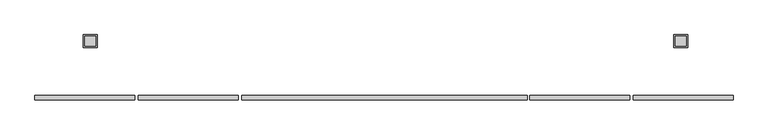
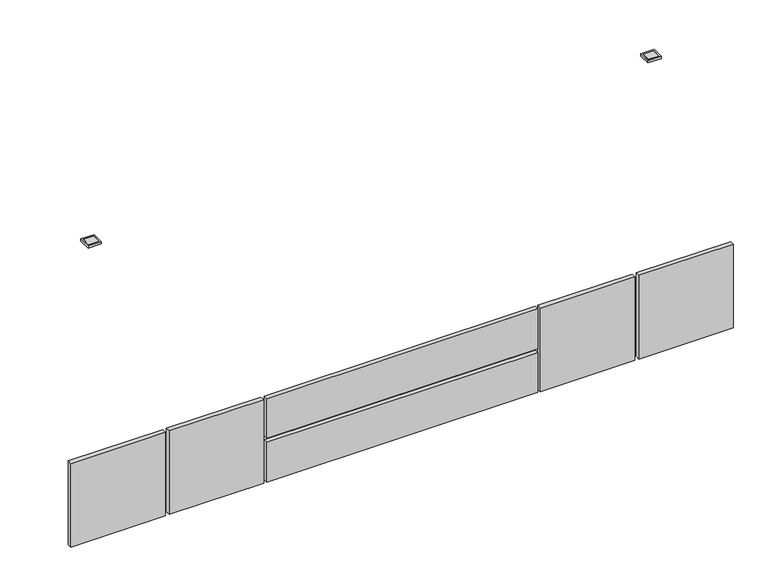
"""IFC4 building model written with IfcOpenShell, lengths in millimetres: furniture geometry."""

from ifc_helpers import new_model, si_unit, frame, origin, place, context, project, spatial, polyline, outline, extrude, source, transform, mapped, element, save


def furniture_15b88f3d(model_context):
    return source(origin(), model_context, "Body", "SweptSolid", [
        extrude(outline(polyline([(1828.0667468, -119.5813198), (1828.0667468, -174.5813198), (1768.0667468, -174.5813198), (1768.0667468, -119.5813198), (1828.0667468, -119.5813198)]), holes=[polyline([(1821.2396229, -126.1492096), (1773.685496, -126.1492096), (1773.685496, -168.0902816), (1821.2396229, -168.0902816), (1821.2396229, -126.1492096)])]), frame((0.0, 0.0, 1436.2366712), z_axis=(0.0, 0.0, 1.0), x_axis=(1.0, 0.0, 0.0)), (0.0, 0.0, 1.0), 10.655453),
        extrude(outline(polyline([(1773.685496, -126.1492096), (1821.2396229, -126.1492096), (1821.2396229, -167.8883204), (1773.685496, -167.8883204), (1773.685496, -126.1492096)])), frame((0.0, 0.0, 1437.5246427), z_axis=(0.0, 0.0, 1.0), x_axis=(1.0, 0.0, 0.0)), (0.0, 0.0, 1.0), 9.3674815),
        extrude(outline(polyline([(1768.0667468, -119.5813198), (1828.0667468, -119.5813198), (1828.0667468, -174.5813198), (1768.0667468, -174.5813198), (1768.0667468, -119.5813198)])), frame((0.0, 0.0, 1444.7177539), z_axis=(0.0, 0.0, 1.0), x_axis=(1.0, 0.0, 0.0)), (0.0, 0.0, 1.0), 2.1743703),
        extrude(outline(polyline([(-708.2110535, -119.5813198), (-708.2110535, -174.5813198), (-768.2110535, -174.5813198), (-768.2110535, -119.5813198), (-708.2110535, -119.5813198)]), holes=[polyline([(-715.0381774, -126.1492096), (-762.5923043, -126.1492096), (-762.5923043, -168.0902816), (-715.0381774, -168.0902816), (-715.0381774, -126.1492096)])]), frame((0.0, 0.0, 1437.3920799), z_axis=(0.0, 0.0, 1.0), x_axis=(1.0, 0.0, 0.0)), (0.0, 0.0, 1.0), 10.655453),
        extrude(outline(polyline([(-762.5923043, -126.1492096), (-715.0381774, -126.1492096), (-715.0381774, -167.8883204), (-762.5923043, -167.8883204), (-762.5923043, -126.1492096)])), frame((0.0, 0.0, 1438.6800514), z_axis=(0.0, 0.0, 1.0), x_axis=(1.0, 0.0, 0.0)), (0.0, 0.0, 1.0), 9.3674815),
        extrude(outline(polyline([(-768.2110535, -119.5813198), (-708.2110535, -119.5813198), (-708.2110535, -174.5813198), (-768.2110535, -174.5813198), (-768.2110535, -119.5813198)])), frame((0.0, 0.0, 1445.8731626), z_axis=(0.0, 0.0, 1.0), x_axis=(1.0, 0.0, 0.0)), (0.0, 0.0, 1.0), 2.1743703),
        extrude(outline(polyline([(-548.829957, -401.0099675), (-976.9610535, -401.0099675), (-976.9610535, -381.0382486), (-548.829957, -381.0382486), (-548.829957, -401.0099675)])), frame((0.0, 0.0, 216.570893), z_axis=(0.0, 0.0, 1.0), x_axis=(1.0, 0.0, 0.0)), (0.0, 0.0, 1.0), 400.0),
        extrude(outline(polyline([(1138.1814975, -401.0099675), (-88.829957, -401.0099675), (-88.829957, -381.0382486), (1138.1814975, -381.0382486), (1138.1814975, -401.0099675)])), frame((0.0, 0.0, 426.570893), z_axis=(0.0, 0.0, 1.0), x_axis=(1.0, 0.0, 0.0)), (0.0, 0.0, 1.0), 190.0),
        extrude(outline(polyline([(1138.1814975, -401.0099675), (-88.829957, -401.0099675), (-88.829957, -381.0382486), (1138.1814975, -381.0382486), (1138.1814975, -401.0099675)])), frame((0.0, 0.0, 216.570893), z_axis=(0.0, 0.0, 1.0), x_axis=(1.0, 0.0, 0.0)), (0.0, 0.0, 1.0), 190.0),
        extrude(outline(polyline([(-103.829957, -401.0099675), (-531.9610535, -401.0099675), (-531.9610535, -381.0382486), (-103.829957, -381.0382486), (-103.829957, -401.0099675)])), frame((0.0, 0.0, 216.570893), z_axis=(0.0, 0.0, 1.0), x_axis=(1.0, 0.0, 0.0)), (0.0, 0.0, 1.0), 400.0),
        extrude(outline(polyline([(2023.0389465, -401.0099675), (1594.9078499, -401.0099675), (1594.9078499, -381.0382486), (2023.0389465, -381.0382486), (2023.0389465, -401.0099675)])), frame((0.0, 0.0, 216.570893), z_axis=(0.0, 0.0, 1.0), x_axis=(1.0, 0.0, 0.0)), (0.0, 0.0, 1.0), 400.0),
        extrude(outline(polyline([(1578.0389465, -401.0099675), (1149.9078499, -401.0099675), (1149.9078499, -381.0382486), (1578.0389465, -381.0382486), (1578.0389465, -401.0099675)])), frame((0.0, 0.0, 216.570893), z_axis=(0.0, 0.0, 1.0), x_axis=(1.0, 0.0, 0.0)), (0.0, 0.0, 1.0), 400.0),
    ])


if __name__ == "__main__":
    model = new_model("IFC4")
    model_context = context("Model", 3, world=origin())
    ifc_project = project(units=[si_unit("LENGTHUNIT", "METRE", prefix="MILLI")], contexts=[model_context])
    site = spatial("IfcSite", under=ifc_project)
    building = spatial("IfcBuilding", under=site)
    placement = place(None, origin())
    furniture_shape = furniture_15b88f3d(model_context)
    element("IfcFurniture", 1, at=placement, inside=building, context=model_context, shape_type="MappedRepresentation", body=[
        mapped(furniture_shape, transform((0.0, 0.0, 0.0), x_axis=(1.0, 0.0, 0.0), y_axis=(0.0, 1.0, 0.0), z_axis=(0.0, 0.0, 1.0))),
    ])
    save(model, "model.ifc")

# Revit data of these elements
# Type
#   Default Elevation = 0
# Element 1 (IfcFurniture)
#   Materials on its faces: "Phase - Demo", "wood 2(1)", "Porcelain, Ivory", "silver", "lit", "Default(1)", "Default Wall", "light", "wood 2", "tv button", "Modern Cabinet", "tv body", "Default", "Poche(1)", "Base Material", "Glass", "gold", "Sculpture"
# Materials
#   "Phase - Demo": class "System", colour RGB 255 255 255, transparency 0, Cost = 0
#   "wood 2(1)": class "Generic", colour RGB 129 75 29, transparency 0, Cost = 0
#   "Porcelain, Ivory": class "Ceramic", colour RGB 120 120 120, transparency 0, Description = "Porcelain, ivory", Cost = 0
#   "silver": class "Generic", colour RGB 120 120 120, transparency 0, Cost = 0
#   "lit": class "Generic", colour RGB 120 120 120, transparency 0, Cost = 0
#   "Default(1)": colour RGB 255 255 255, transparency 0, Cost = 0
#   "Default Wall": colour RGB 255 255 255, transparency 0, Cost = 0
#   "light": colour RGB 127 127 127, transparency 0, Cost = 0
#   "wood 2": class "Generic", colour RGB 120 120 120, transparency 0, Cost = 0
#   "tv button": class "Generic", colour RGB 120 120 120, transparency 0, Cost = 0
#   "Modern Cabinet": colour RGB 143 95 62, transparency 0, Cost = 0
#   "tv body": class "System", colour RGB 0 0 255, transparency 0, Cost = 0
#   "Default": colour RGB 255 255 255, transparency 0
#   "Poche(1)": class "System", colour RGB 244 244 244, transparency 0, Cost = 0
#   "Base Material": class "Glass", colour RGB 172 172 172, transparency 0, Cost = 0
#   "Glass": class "Glass", colour RGB 218 227 224, transparency 0.85, Description = "Soda Lime Glass", Cost = 0
#   "gold": class "Generic", colour RGB 120 120 120, transparency 0, Cost = 0
#   "Sculpture": colour RGB 219 183 111, transparency 0, Cost = 0
